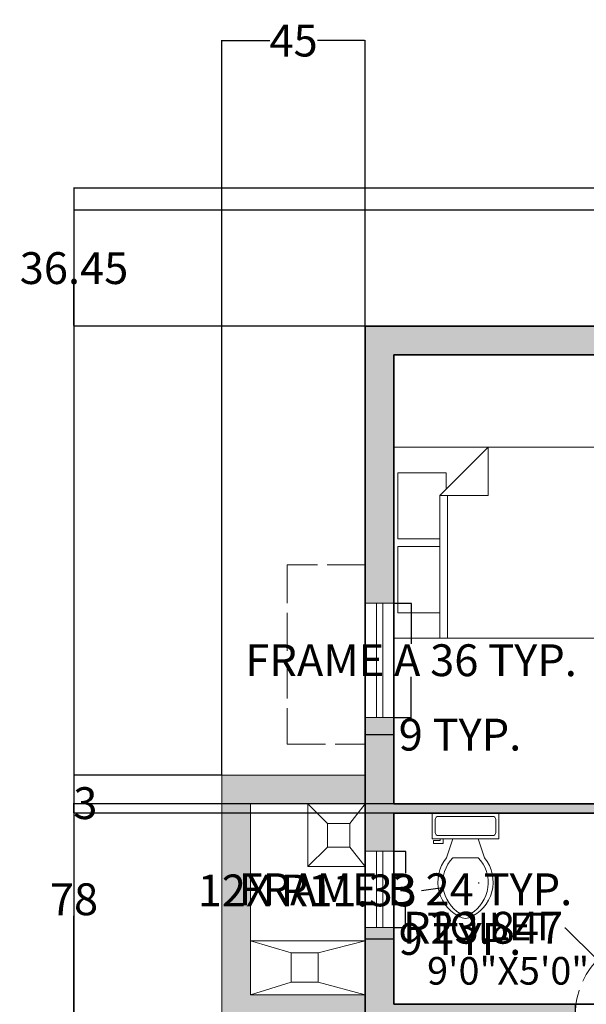
# Model space of a CAD drawing. Units: inches. Extents: x 215 to 969, y -612 to 418.
# Tile 5 of 8: x 227 to 405, y 109 to 418. Entities that reach past the tile are written whole.
import ezdxf

# ---------------------------------------------------------------- set-up
doc = ezdxf.new("R2010")
doc.units = ezdxf.units.IN
doc.header["$MEASUREMENT"] = 0
doc.linetypes.add('ACAD_ISO02W100', pattern=[15, 12, -3])
for name, color, linetype, lineweight in [('A-ANNO-DIMS', 2, 'Continuous', 18), ('A-AREA-IDEN', 7, 'Continuous', 18), ('A-DOOR', 3, 'Continuous', 25), ('A-DOOR-SWNG', 3, 'ACAD_ISO02W100', 13), ('A-FLOR-FIXT', 9, 'Continuous', 18), ('A-FLOR-OVHD', 8, 'ACAD_ISO02W100', 13), ('A-FLOR-SHFT', 9, 'Continuous', 18), ('A-FURN', 8, 'Continuous', 18), ('A-GLAZ', 4, 'Continuous', 18), ('A-WALL', 7, 'Continuous', 35)]:
    doc.layers.add(name, color=color, linetype=linetype, lineweight=lineweight)
doc.layers.add('A-WALL-PATT', color=252, linetype='Continuous', lineweight=13, true_color=0x939598)
doc.styles.get("Standard").update_dxf_attribs({"font": 'arial.ttf'})
doc.dimstyles.get("Standard").update_dxf_attribs({"dimtxt": 10, "dimasz": 0.18, "dimexe": 0.18, "dimexo": 0.0625, "dimgap": 0.09, "dimtad": 0, "dimtih": 1, "dimtoh": 1, "dimdec": 0, "dimzin": 0, "dimdsep": 46, "dimlunit": 3, "dimtxsty": 'Standard', "dimcen": 0.09, "dimadec": 0, "dimazin": 0, "dimtfac": 1, "dimtdec": 0, "dimtofl": 0, "dimtmove": 0, "dimatfit": 3, "dimfxl": 1, "dimtolj": 1, "dimtzin": 0, "dimarcsym": 0})

# ---------------------------------------------------------------- blocks, each defined once
blk = doc.blocks.new('Bed - Queen')
for p, q in [((0, -80.00003), (0, 0)), ((0, 0), (59.99999, 0)), ((59.99999, 0), (59.99999, -80.00003)), ((7.99999, -1.2), (28.79998, -1.2)), ((7.99999, -14.4), (7.99999, -1.2)), ((28.79998, -1.2), (28.79998, -14.4)), ((31.19999, -1.2), (51.99999, -1.2)), ((31.19999, -14.4), (31.19999, -1.2)), ((51.99999, -1.2), (51.99999, -16.4)), ((0, -14.4), (44.8, -14.4)), ((59.99999, -29.6), (44.8, -14.4)), ((44.8, -14.4), (44.8, -29.6)), ((44.8, -16.8), (0, -16.8)), ((51.99999, -16.4), (46.79936, -16.4)), ((44.8, -29.6), (59.99999, -29.6)), ((59.99999, -80.00003), (0, -80.00003))]:
    blk.add_line(p, q)
blk = doc.blocks.new('Toilet - top')
for p, q in [((9.5, -6), (9.5, -2)), ((-10, -8.5), (-8, -8.5)), ((-10, -9.5), (-10, -8.5)), ((-8, -8.5), (-8, -8)), ((-7, -8), (-7, -9.5)), ((-4, -8), (-6, -14)), ((4, -8), (6, -14)), ((-7, -9.5), (-10, -9.5)), ((4, -14), (-4, -14))]:
    blk.add_line(p, q)
blk.add_lwpolyline([(10.5, -8), (10.5, 0), (-10.5, 0), (-10.5, -8)], close=True)
for points in [[(-9.5, -2), (-9.5, -6)], [(8.5, -1), (-8.5, -1)], [(-8.5, -7), (8.5, -7)]]:
    blk.add_lwpolyline(points)
for centre, radius, start, end in [((-8.62, -1.88), 0.884, 81.8699, 188.1301), ((8.62, -1.88), 0.884, 351.8699, 98.1301), ((-8.62, -6.12), 0.884, 171.8699, 278.1301), ((8.62, -6.12), 0.884, 261.8699, 8.1301), ((3.52, -21.58), 12.17, 141.4691, 247.9714), ((4.2, -21.82), 11.33, 136.3677, 238.9468), ((-3.52, -21.58), 12.17, 292.0284, 38.5307), ((-4.2, -21.82), 11.33, 301.053, 43.6321), ((0, -27.88), 4, 245.7318, 294.2682), ((0, -29), 4, 254.8605, 285.1395)]:
    blk.add_arc(centre, radius, start, end)
blk = doc.blocks.new('WINDOW-SHADE-56')
for p, q in [((24.46, 56.34), (0, 56.34)), ((0, 56.34), (0, 0)), ((0, 0), (24.46, 0))]:
    blk.add_line(p, q)
blk = doc.blocks.new('WIN-FRAME-24B')
for p, q in [((0, 23.99), (9, 23.99)), ((3.5, 23.99), (3.5, 0)), ((5.5, 23.99), (5.5, 0)), ((9, 0), (0, 0)), ((4.5, 0), (9, 0))]:
    blk.add_line(p, q)
blk = doc.blocks.new('WIN-FRAME-36A')
for p, q in [((0, 35.94), (9, 35.94)), ((3.5, 35.94), (3.5, 0)), ((5.5, 35.94), (5.5, 0)), ((9, 0), (0, 0)), ((4.5, 0), (9, 0))]:
    blk.add_line(p, q)
blk = doc.blocks.new('*D41')
at = {"layer": 'A-ANNO-DIMS', "color": 0, "lineweight": -2, "transparency": 16777216}
for p, q in [((344.42, 235.25), (349.92, 235.25)), ((349.74, 235.07), (349.74, 222.48)), ((349.74, 199.49), (349.74, 212.08)), ((344.42, 199.31), (349.92, 199.31))]:
    blk.add_line(p, q, dxfattribs=at)
at = {"layer": 'A-ANNO-DIMS', "color": 0, "transparency": 16777216}
for points in [[(349.71, 235.07), (349.77, 235.07), (349.74, 235.25)], [(349.71, 199.49), (349.77, 199.49), (349.74, 199.31)]]:
    blk.add_solid(points, dxfattribs=at)
at = {"layer": 'Defpoints', "color": 0, "transparency": 16777216}
for p in [(344.35, 235.25), (349.74, 235.25), (344.35, 199.31)]:
    blk.add_point(p, dxfattribs=at)
at = {"layer": 'A-ANNO-DIMS', "color": 0, "transparency": 16777216, "insert": (349.74, 217.28), "char_height": 10, "attachment_point": 5}
blk.add_mtext('\\A1;FRAME A 36 TYP.', dxfattribs=at)
blk = doc.blocks.new('*D42')
at = {"layer": 'A-ANNO-DIMS', "color": 0, "lineweight": -2, "transparency": 16777216}
for p, q in [((335.35, 199.25), (335.35, 193.74)), ((344.35, 199.25), (344.35, 193.74)), ((335.53, 193.92), (344.17, 193.92)), ((344.35, 193.92), (344.53, 193.92))]:
    blk.add_line(p, q, dxfattribs=at)
at = {"layer": 'A-ANNO-DIMS', "color": 0, "transparency": 16777216}
for points in [[(335.53, 193.95), (335.53, 193.89), (335.35, 193.92)], [(344.17, 193.95), (344.17, 193.89), (344.35, 193.92)]]:
    blk.add_solid(points, dxfattribs=at)
at = {"layer": 'Defpoints', "color": 0, "transparency": 16777216}
for p in [(335.35, 199.31), (344.35, 199.31), (344.35, 193.92)]:
    blk.add_point(p, dxfattribs=at)
at = {"layer": 'A-ANNO-DIMS', "color": 0, "transparency": 16777216, "insert": (365.08, 193.92), "char_height": 10, "attachment_point": 5}
blk.add_mtext('\\A1;9 TYP.', dxfattribs=at)
blk = doc.blocks.new('*D47')
at = {"layer": 'A-ANNO-DIMS', "color": 0, "lineweight": -2, "transparency": 16777216}
for p, q in [((344.42, 157.34), (348.13, 157.34)), ((347.95, 157.16), (347.95, 150.45)), ((347.95, 133.52), (347.95, 140.23)), ((344.42, 133.34), (348.13, 133.34))]:
    blk.add_line(p, q, dxfattribs=at)
at = {"layer": 'A-ANNO-DIMS', "color": 0, "transparency": 16777216}
for points in [[(347.92, 157.16), (347.98, 157.16), (347.95, 157.34)], [(347.92, 133.52), (347.98, 133.52), (347.95, 133.34)]]:
    blk.add_solid(points, dxfattribs=at)
at = {"layer": 'Defpoints', "color": 0, "transparency": 16777216}
for p in [(344.35, 157.34), (347.95, 157.34), (344.35, 133.34)]:
    blk.add_point(p, dxfattribs=at)
at = {"layer": 'A-ANNO-DIMS', "color": 0, "transparency": 16777216, "insert": (347.95, 145.34), "char_height": 10, "attachment_point": 5}
blk.add_mtext('\\A1;FRAME B 24 TYP.', dxfattribs=at)
blk = doc.blocks.new('*D48')
at = {"layer": 'A-ANNO-DIMS', "color": 0, "lineweight": -2, "transparency": 16777216}
for p, q in [((335.35, 133.28), (335.35, 129.57)), ((344.35, 133.28), (344.35, 129.57)), ((335.53, 129.75), (344.17, 129.75)), ((344.35, 129.75), (344.53, 129.75))]:
    blk.add_line(p, q, dxfattribs=at)
at = {"layer": 'A-ANNO-DIMS', "color": 0, "transparency": 16777216}
for points in [[(335.53, 129.78), (335.53, 129.72), (335.35, 129.75)], [(344.17, 129.78), (344.17, 129.72), (344.35, 129.75)]]:
    blk.add_solid(points, dxfattribs=at)
at = {"layer": 'Defpoints', "color": 0, "transparency": 16777216}
for p in [(335.35, 133.34), (344.35, 133.34), (344.35, 129.75)]:
    blk.add_point(p, dxfattribs=at)
at = {"layer": 'A-ANNO-DIMS', "color": 0, "transparency": 16777216, "insert": (365.08, 129.75), "char_height": 10, "attachment_point": 5}
blk.add_mtext('\\A1;9 TYP.', dxfattribs=at)
blk = doc.blocks.new('*D73')
at = {"layer": 'A-ANNO-DIMS', "color": 0, "lineweight": -2, "transparency": 16777216}
for p, q in [((290.35, 181.28), (290.35, 412.08)), ((290.53, 411.9), (305.36, 411.9)), ((335.17, 411.9), (320.34, 411.9)), ((335.35, 181.28), (335.35, 412.08))]:
    blk.add_line(p, q, dxfattribs=at)
at = {"layer": 'A-ANNO-DIMS', "color": 0, "transparency": 16777216}
for points in [[(290.53, 411.93), (290.53, 411.87), (290.35, 411.9)], [(335.17, 411.93), (335.17, 411.87), (335.35, 411.9)]]:
    blk.add_solid(points, dxfattribs=at)
at = {"layer": 'Defpoints', "color": 0, "transparency": 16777216}
for p in [(335.35, 411.9), (290.35, 181.21), (335.35, 181.21)]:
    blk.add_point(p, dxfattribs=at)
at = {"layer": 'A-ANNO-DIMS', "color": 0, "transparency": 16777216, "insert": (312.85, 411.9), "char_height": 10, "attachment_point": 5}
blk.add_mtext('\\A1;45', dxfattribs=at)
blk = doc.blocks.new('*D74')
at = {"layer": 'A-ANNO-DIMS', "color": 0, "lineweight": -2, "transparency": 16777216}
for p, q in [((290.29, 181.21), (243.77, 181.21)), ((243.95, 181.03), (243.95, 147.41)), ((243.95, 103.39), (243.95, 137.02)), ((290.29, 103.21), (243.77, 103.21))]:
    blk.add_line(p, q, dxfattribs=at)
at = {"layer": 'A-ANNO-DIMS', "color": 0, "transparency": 16777216}
for points in [[(243.92, 181.03), (243.98, 181.03), (243.95, 181.21)], [(243.92, 103.39), (243.98, 103.39), (243.95, 103.21)]]:
    blk.add_solid(points, dxfattribs=at)
at = {"layer": 'Defpoints', "color": 0, "transparency": 16777216}
for p in [(243.95, 181.21), (290.35, 181.21), (290.35, 103.21)]:
    blk.add_point(p, dxfattribs=at)
at = {"layer": 'A-ANNO-DIMS', "color": 0, "transparency": 16777216, "insert": (243.95, 142.21), "char_height": 10, "attachment_point": 5}
blk.add_mtext('\\A1;78', dxfattribs=at)
blk = doc.blocks.new('*D76')
at = {"layer": 'A-ANNO-DIMS', "color": 0, "lineweight": -2, "transparency": 16777216}
for p, q in [((569.29, 365.5), (243.77, 365.5)), ((243.95, 365.32), (243.95, -91.71)), ((243.95, -559.13), (243.95, -102.1)), ((454.66, -559.31), (243.77, -559.31))]:
    blk.add_line(p, q, dxfattribs=at)
at = {"layer": 'A-ANNO-DIMS', "color": 0, "transparency": 16777216}
for points in [[(243.92, 365.32), (243.98, 365.32), (243.95, 365.5)], [(243.92, -559.13), (243.98, -559.13), (243.95, -559.31)]]:
    blk.add_solid(points, dxfattribs=at)
at = {"layer": 'Defpoints', "color": 0, "transparency": 16777216}
for p in [(569.35, 365.5), (243.95, -559.31), (454.72, -559.31)]:
    blk.add_point(p, dxfattribs=at)
at = {"layer": 'A-ANNO-DIMS', "color": 0, "transparency": 16777216, "insert": (243.95, -96.91), "char_height": 10, "attachment_point": 5}
blk.add_mtext('\\A1;924.8', dxfattribs=at)
blk = doc.blocks.new('*D78')
at = {"layer": 'A-ANNO-DIMS', "color": 0, "lineweight": -2, "transparency": 16777216}
for p, q in [((503.29, 358.66), (243.77, 358.66)), ((243.95, 358.48), (243.95, 345.64)), ((243.95, 322.39), (243.95, 335.24)), ((503.29, 322.21), (243.77, 322.21))]:
    blk.add_line(p, q, dxfattribs=at)
at = {"layer": 'A-ANNO-DIMS', "color": 0, "transparency": 16777216}
for points in [[(243.92, 358.48), (243.98, 358.48), (243.95, 358.66)], [(243.92, 322.39), (243.98, 322.39), (243.95, 322.21)]]:
    blk.add_solid(points, dxfattribs=at)
at = {"layer": 'Defpoints', "color": 0, "transparency": 16777216}
for p in [(503.35, 358.66), (243.95, 322.21), (503.35, 322.21)]:
    blk.add_point(p, dxfattribs=at)
at = {"layer": 'A-ANNO-DIMS', "color": 0, "transparency": 16777216, "insert": (243.95, 340.44), "char_height": 10, "attachment_point": 5}
blk.add_mtext('\\A1;36.45', dxfattribs=at)
blk = doc.blocks.new('*D83')
at = {"layer": 'A-ANNO-DIMS', "color": 0, "lineweight": -2, "transparency": 16777216}
for p, q in [((344.29, 172.21), (243.77, 172.21)), ((243.95, 172.21), (243.95, 172.39)), ((243.95, 172.39), (244.13, 172.39)), ((243.95, 169.39), (243.95, 172.03)), ((344.29, 169.21), (243.77, 169.21))]:
    blk.add_line(p, q, dxfattribs=at)
at = {"layer": 'A-ANNO-DIMS', "color": 0, "transparency": 16777216}
for points in [[(243.92, 172.03), (243.98, 172.03), (243.95, 172.21)], [(243.92, 169.39), (243.98, 169.39), (243.95, 169.21)]]:
    blk.add_solid(points, dxfattribs=at)
at = {"layer": 'Defpoints', "color": 0, "transparency": 16777216}
for p in [(243.95, 172.21), (344.35, 172.21), (344.35, 169.21)]:
    blk.add_point(p, dxfattribs=at)
at = {"layer": 'A-ANNO-DIMS', "color": 0, "transparency": 16777216, "insert": (247.5, 172.39), "char_height": 10, "attachment_point": 5}
blk.add_mtext('\\A1;3', dxfattribs=at)
blk = doc.blocks.new('*D85')
at = {"layer": 'A-ANNO-DIMS', "color": 0, "lineweight": -2, "transparency": 16777216}
for p, q in [((397.96, 133.26), (398.14, 133.26)), ((398.14, 133.26), (408.16, 123.3)), ((425.11, 106.37), (425.29, 106.37)), ((425.2, 106.28), (425.2, 106.46))]:
    blk.add_line(p, q, dxfattribs=at)
at = {"layer": 'A-ANNO-DIMS', "color": 0, "transparency": 16777216}
blk.add_solid([(408.18, 123.32), (408.14, 123.28), (408.29, 123.18)], dxfattribs=at)
at = {"layer": 'Defpoints', "color": 0, "transparency": 16777216}
for p in [(408.29, 123.18), (425.2, 106.37)]:
    blk.add_point(p, dxfattribs=at)
at = {"layer": 'A-ANNO-DIMS', "color": 0, "transparency": 16777216, "insert": (372.32, 133.26), "char_height": 10, "attachment_point": 5}
blk.add_mtext('\\A1;R23.847', dxfattribs=at)
blk = doc.blocks.new('*D96')
at = {"layer": 'A-ANNO-DIMS', "color": 0, "lineweight": -2, "transparency": 16777216}
for p, q in [((353.05, 144.98), (359.61, 145.86)), ((370.93, 147.4), (371.11, 147.4)), ((371.02, 147.31), (371.02, 147.49))]:
    blk.add_line(p, q, dxfattribs=at)
at = {"layer": 'A-ANNO-DIMS', "color": 0, "transparency": 16777216}
blk.add_solid([(359.61, 145.89), (359.62, 145.83), (359.79, 145.88)], dxfattribs=at)
at = {"layer": 'Defpoints', "color": 0, "transparency": 16777216}
for p in [(359.79, 145.88), (371.02, 147.4)]:
    blk.add_point(p, dxfattribs=at)
at = {"layer": 'A-ANNO-DIMS', "color": 0, "transparency": 16777216, "insert": (317.15, 144.98), "char_height": 10, "attachment_point": 5}
blk.add_mtext('\\A1;12X R11.33', dxfattribs=at)

msp = doc.modelspace()

# ---------------------------------------------------------------- hatches: boundary and pattern name
at = {"layer": 'A-WALL-PATT'}
h = msp.add_hatch(color=256, dxfattribs=at)
h.dxf.hatch_style = 1
h.paths.add_polyline_path([(764.0736, 322.2135), (569.3535, 322.2135), (565.0643, 322.2135), (565.0643, 313.2135), (569.3535, 313.2135), (569.3535, 205.2135), (509.3535, 205.2135), (509.3535, 247.2592), (506.3535, 247.2592), (506.3535, 172.2135), (491.3535, 172.2135), (491.3535, 169.2135), (509.3535, 169.2135), (509.3535, 202.2135), (569.3535, 202.2135), (569.3535, 169.2135), (578.3535, 169.2135), (578.3535, 205.2135), (578.3535, 237.2135), (615.7789, 237.2135), (615.7789, 246.2135), (578.3535, 246.2135), (578.3535, 313.2135), (710.3535, 313.2135), (710.3535, 246.2135), (710.3535, 211.3874), (719.3535, 211.3874), (719.3535, 295.2135), (719.3535, 313.2135), (764.0736, 313.2135)])
h.paths.add_polyline_path([(879.3535, 322.2135), (811.6486, 322.2135), (811.6486, 313.2135), (870.3535, 313.2135), (870.3535, 215.3905, -0.06325422), (879.3535, 216.5337), (879.3535, 313.2135)])
h.paths.add_polyline_path([(879.3535, 157.2135), (879.3535, 180.5337), (870.3535, 180.5337), (870.3535, 157.2135), (719.3535, 157.2135), (710.3535, 157.2135), (710.3535, 148.2135), (719.3535, 148.2135), (870.3535, 148.2135), (870.3535, 16.2135), (838.4933, 16.2135), (838.4933, 13.2135), (870.3535, 13.2135), (870.3535, -37.7865), (844.0345, -37.7865), (844.0345, -46.7865), (870.3535, -46.7865), (879.3535, -46.7865), (879.3535, -37.7865), (879.3535, 137.613)])
h.paths.add_polyline_path([(710.3535, 246.2135), (663.4146, 246.2135), (663.4146, 237.2135), (710.3535, 237.2135)], flags=17)
h.paths.add_polyline_path([(541.2942, 322.2135), (509.3535, 322.2135), (468.3222, 322.2135), (468.3222, 313.2135), (500.3535, 313.2135), (509.3535, 313.2135), (541.2942, 313.2135)])
h.paths.add_polyline_path([(509.3535, 313.2135), (503.3535, 313.2135), (503.3535, 277.5241, -0.04952579), (509.3535, 277.4203)], flags=17)
h.paths.add_polyline_path([(420.2828, 322.2135), (335.3535, 322.2135), (335.3535, 235.2487), (344.3535, 235.2487), (344.3535, 284.1885), (344.3535, 313.2135), (420.2828, 313.2135)])
h.paths.add_polyline_path([(335.3535, 181.2135), (290.3535, 181.2135), (290.3535, 103.2135), (335.3535, 103.2135), (335.3535, 112.2135), (299.3535, 112.2135), (299.3535, 129.1615), (299.3535, 172.2135), (335.3535, 172.2135)])
h.paths.add_polyline_path([(344.3535, 199.3097), (335.3535, 199.3097), (335.3535, 172.2135), (335.3535, 157.3369), (344.3535, 157.3369), (344.3535, 169.2135), (452.3535, 169.2135), (452.5037, 169.2135), (452.5037, 150.1199), (452.3535, 109.2135), (455.3535, 109.2135), (455.3535, 169.2135, -0.02086055), (455.4787, 172.2135), (344.3535, 172.2135)])
h.paths.add_polyline_path([(344.3535, 133.3441), (335.3535, 133.3441), (335.3535, 77.89), (344.3535, 77.89), (344.3535, 103.2135), (401.3556, 103.2135), (401.3556, 109.2135), (344.3535, 109.2135)])
h.paths.add_polyline_path([(462.6362, 109.2135), (443.0437, 109.2135), (425.2018, 109.2135), (425.2018, 106.2135), (452.3535, 106.2135), (462.7615, 106.2135, -0.02086055)])
h.paths.add_polyline_path([(540.3535, 106.2135), (684.3535, 106.2135), (684.3535, 35.7135), (687.3535, 35.7135), (687.3535, 56.1856), (693.3535, 56.1856), (693.3535, 109.2135), (540.3535, 109.2135), (531.3535, 109.2135), (498.6362, 109.2135), (498.6362, 106.2135), (531.3535, 106.2135), (531.3535, -37.7865), (507.9524, -37.7865), (507.9524, -46.7865), (610.6038, -46.7865), (610.6038, -37.7865), (540.3535, -37.7865)])
h.paths.add_polyline_path([(578.3535, 358.6622), (555.879, 358.6622), (555.879, 349.6622), (569.3535, 349.6622), (569.3535, 322.2135), (578.3535, 322.2135)])
h.paths.add_polyline_path([(525.962, 358.6622), (503.3535, 358.6622), (503.3535, 322.2135), (509.3535, 322.2135), (509.3535, 349.6622), (525.962, 349.6622)])
h.paths.add_polyline_path([(344.3535, 30.022), (335.3535, 30.022), (335.3535, -37.7865), (335.3535, -46.7865), (484.3302, -46.7865), (484.3302, -37.7865), (344.3535, -37.7865)])
h.paths.add_polyline_path([(719.1188, -37.7865), (698.4193, -37.7865), (693.3535, -37.7865), (693.3535, 7.424, -0.07717369), (684.3535, 6.0404), (684.3535, -37.7865), (658.8269, -37.7865), (658.8269, -46.7865), (684.3535, -46.7865), (684.3535, -82.7865), (693.3535, -82.7865), (704.1236, -82.7865), (704.1236, -78.0462), (693.3535, -78.0462), (693.3535, -46.7865), (719.1188, -46.7865)])
h.paths.add_polyline_path([(684.3535, -14.2202), (669.6716, -14.2202), (669.6716, -16.6044, -0.23606798), (667.6716, -17.6044), (667.6716, -18.6044, -0.11764706), (650.6716, -18.6044), (650.6716, -17.6044, -0.23606798), (648.6716, -16.6044), (648.6716, -14.2202), (603.0565, -14.2202), (603.0565, -37.7865), (684.3535, -37.7865)], flags=17)
h.paths.add_polyline_path([(665.6716, -14.2202), (652.6716, -14.2202), (652.6716, -16.6044, -0.23606798), (650.6716, -17.6044), (650.6716, -18.6044, 0.11764706), (667.6716, -18.6044), (667.6716, -17.6044, -0.23606798), (665.6716, -16.6044)], flags=16)
h.paths.add_polyline_path([(786.7385, -37.7865), (755.3535, -37.7865), (755.3535, 13.2135), (769.0808, 13.2135), (769.0808, 16.2135), (755.3535, 16.2135), (755.3535, 73.2135), (753.3535, 73.2135), (693.3535, 73.2135), (693.3535, 70.2135), (753.3535, 70.2135), (753.3535, -37.7865), (743.3062, -37.7865), (743.3062, -46.7865), (781.7385, -46.7865), (781.7385, -82.7865), (786.7385, -82.7865), (786.7385, -82.3744), (786.7385, -46.7865)])
h.paths.add_polyline_path([(844.0345, -37.7865), (786.7385, -37.7865), (786.7385, -46.7865), (844.0345, -46.7865)], flags=17)
h.paths.add_polyline_path([(781.7385, -78.0462), (704.1236, -78.0462), (704.1236, -82.7865), (781.7385, -82.7865)], flags=17)
h.paths.add_polyline_path([(344.3535, -46.7865), (335.3535, -46.7865), (335.3535, -166.4525), (344.3535, -166.4525)])
h.paths.add_polyline_path([(382.6632, 103.2135), (344.3535, 103.2135), (344.3535, 77.89), (344.3535, 32.7135), (363.5083, 32.7135), (382.6632, 32.7135)])
h.paths.add_polyline_path([(879.3535, -46.7865), (870.3535, -46.7865), (870.3535, -166.4525), (879.3535, -166.4525)])
h.paths.add_polyline_path([(879.3535, -166.4525), (799.4745, -166.4525), (799.4745, -175.4525), (855.3535, -175.4525), (870.3535, -175.4525), (870.3535, -192.5449), (879.3535, -192.5449), (879.3535, -175.4525)])
h.paths.add_polyline_path([(763.1775, -166.4525), (655.7214, -166.4525), (655.7214, -175.4525), (763.1775, -175.4525)])
h.paths.add_polyline_path([(619.8538, -166.4525), (550.8369, -166.4525), (550.8369, -175.4525), (619.8538, -175.4525)])
h.paths.add_polyline_path([(527.1282, -166.4525), (427.0819, -166.4525), (427.0819, -175.4525), (527.1282, -175.4525)])
h.paths.add_polyline_path([(391.4021, -166.4525), (335.3535, -166.4525), (335.3535, -175.4525), (335.3535, -236.0109), (344.3535, -236.0109), (344.3535, -187.5037), (344.3535, -175.4525), (391.4021, -175.4525)])
h.paths.add_polyline_path([(344.3535, -271.9249), (335.3535, -271.9249), (335.3535, -331.0209), (344.3535, -331.0209), (344.3535, -314.4525), (412.4218, -314.4525, -0.02503209), (412.3073, -311.4525), (344.3535, -311.4525)])
h.paths.add_polyline_path([(470.1954, -311.4525), (442.3073, -311.4525), (442.3073, -314.4525), (470.0702, -314.4525, -0.02086055)])
h.paths.add_polyline_path([(455.3535, -314.4525), (452.3535, -314.4525), (452.3535, -374.4525), (455.3535, -374.4525)])
h.paths.add_polyline_path([(579.3535, -241.4072), (519.3535, -241.4072), (519.3535, -283.4525), (579.3535, -283.4525)])
h.paths.add_polyline_path([(516.5043, -281.1089), (584.3098, -281.1089), (584.3098, -264.0138), (516.5043, -264.0138)], flags=9)
h.paths.add_polyline_path([(516.4662, -263.2183), (581.1504, -263.2183), (581.1504, -245.8948), (516.4662, -245.8948)], flags=9)

# ---------------------------------------------------------------- linework, layer by layer
at = {"layer": 'A-DOOR'}
msp.add_line((401.3556, 103.2135), (401.3556, 109.2135), dxfattribs=at)
at = {"layer": 'A-DOOR-SWNG'}
msp.add_arc((425.2018, 106.3669), 23.8466, 90, 180.368506, dxfattribs=at)
at = {"layer": 'A-FLOR-SHFT'}
for p, q in [((290.3535, 181.2135), (290.3535, 103.2135)), ((335.3535, 181.2135), (290.3535, 181.2135)), ((335.3535, 172.2135), (299.3535, 172.2135)), ((299.3535, 172.2135), (299.3535, 112.2135)), ((323.4787, 166.0316), (317.3245, 172.2135)), ((330.538, 166.0316), (335.3535, 172.2135)), ((323.4787, 158.6192), (317.3245, 152.4723)), ((330.538, 158.6192), (335.3535, 152.4723)), ((312.1553, 125.4125), (299.3535, 129.1615)), ((320.5486, 125.4125), (335.3535, 129.1615)), ((312.1553, 116.1621), (299.3535, 112.2135)), ((320.5486, 116.1621), (335.3535, 112.2135)), ((299.3535, 112.2135), (335.3535, 112.2135))]:
    msp.add_line(p, q, dxfattribs=at)
for points in [[(335.3535, 172.2135), (317.3245, 172.2135), (317.3245, 152.4723), (335.3535, 152.4723)], [(323.4787, 166.0316), (330.538, 166.0316), (330.538, 158.6192), (323.4787, 158.6192)], [(335.3535, 112.2135), (299.3535, 112.2135), (299.3535, 129.1615), (335.3535, 129.1615)], [(312.1553, 125.4125), (320.5486, 125.4125), (320.5486, 116.1621), (312.1553, 116.1621)]]:
    msp.add_lwpolyline(points, close=True, dxfattribs=at)
at = {"layer": 'A-WALL'}
for p, q in [((335.3535, 322.2135), (509.3535, 322.2135)), ((335.3535, 322.2135), (335.3535, 172.2135)), ((344.3535, 313.2135), (500.3535, 313.2135)), ((344.3535, 313.2135), (344.3535, 172.2135)), ((335.3535, -37.7865), (335.3535, 172.2135)), ((344.3535, 172.2135), (455.4787, 172.2135)), ((335.3535, 169.2135), (335.3535, 109.2135)), ((344.3535, 169.2135), (452.3535, 169.2135)), ((344.3535, 169.2135), (344.3535, 109.2135)), ((344.3535, 109.2135), (452.3535, 109.2135))]:
    msp.add_line(p, q, dxfattribs=at)

# ---------------------------------------------------------------- block references
at = {"layer": 'A-FLOR-FIXT'}
msp.add_blockref('Toilet - top', (366.8192, 169.2135), dxfattribs=at)
at = {"layer": 'A-FLOR-OVHD'}
msp.add_blockref('WINDOW-SHADE-56', (310.895, 190.878), dxfattribs=at)
at = {"layer": 'A-FURN', "rotation": 90}
msp.add_blockref('Bed - Queen', (344.3535, 224.1885), dxfattribs=at)
at = {"layer": 'A-GLAZ'}
for name, p in [('WIN-FRAME-36A', (335.353, 199.31)), ('WIN-FRAME-24B', (335.353, 133.344))]:
    msp.add_blockref(name, p, dxfattribs=at)

# ---------------------------------------------------------------- texts
at = {"layer": 'A-AREA-IDEN'}
for s, p in [('TOILET', (354.7688, 129.3376)), ('9\'0"X5\'0"', (354.7688, 115.3982))]:
    msp.add_text(s, height=8.67737, dxfattribs=at).set_placement(p)

# ---------------------------------------------------------------- dimensions: what is measured, and where the dimension line sits
at = {"layer": 'A-ANNO-DIMS'}
dim = msp.add_linear_dim(base=(335.3535, 411.9008), p1=(290.3535, 181.2135), p2=(335.3535, 181.2135), dimstyle='Standard', override={"dimdec": 0, "dimlfac": 1, "dimrnd": 0, "dimzin": 0, "dimdsep": 46, "dimlunit": 2}, dxfattribs=at)
dim.commit()
dim.dimension.update_dxf_attribs({"geometry": '*D73', "text_midpoint": (312.8535, 411.9008)})
for base, p1, p2, override, picture, middle in [((243.9535, -559.3132), (569.3535, 365.5008), (454.7218, -559.3132), {"dimdec": 1, "dimlfac": 1, "dimrnd": 0, "dimzin": 0, "dimdsep": 46, "dimlunit": 2}, '*D76', (243.9535, -96.9062)), ((243.9535, 322.2135), (503.3535, 358.6622), (503.3535, 322.2135), {"dimdec": 2, "dimlfac": 1, "dimrnd": 0, "dimzin": 0, "dimdsep": 46, "dimlunit": 2}, '*D78', (243.9535, 340.4379)), ((243.9535, 181.2135), (290.3535, 103.2135), (290.3535, 181.2135), {"dimdec": 0, "dimlfac": 1, "dimrnd": 0, "dimzin": 0, "dimdsep": 46, "dimlunit": 2}, '*D74', (243.9535, 142.2135)), ((243.9535, 172.2135), (344.3535, 169.2135), (344.3535, 172.2135), {"dimdec": 0, "dimlfac": 1, "dimrnd": 0, "dimzin": 0, "dimdsep": 46, "dimlunit": 2}, '*D83', (247.4977, 172.3935))]:
    dim = msp.add_linear_dim(base=base, p1=p1, p2=p2, angle=90, dimstyle='Standard', override=override, dxfattribs=at)
    dim.commit()
    dim.dimension.update_dxf_attribs({"geometry": picture, "text_midpoint": middle})
for base, p1, p2, text, picture, middle in [((349.7443, 235.2487), (344.3535, 199.3097), (344.3535, 235.2487), 'FRAME A <> TYP.', '*D41', (349.7443, 217.2792)), ((347.9524, 157.3369), (344.3535, 133.3441), (344.3535, 157.3369), 'FRAME B <> TYP.', '*D47', (347.9524, 145.3405))]:
    dim = msp.add_linear_dim(base=base, p1=p1, p2=p2, angle=90, text=text, dimstyle='Standard', override={"dimdec": 0, "dimlfac": 1, "dimrnd": 0, "dimzin": 0, "dimdsep": 46, "dimlunit": 2}, dxfattribs=at)
    dim.commit()
    dim.dimension.update_dxf_attribs({"geometry": picture, "text_midpoint": middle})
for base, p1, p2, picture, middle in [((344.3535, 193.9188), (335.3535, 199.3097), (344.3535, 199.3097), '*D42', (365.0771, 193.9188)), ((344.3535, 129.7452), (335.3535, 133.3441), (344.3535, 133.3441), '*D48', (365.0771, 129.7452))]:
    dim = msp.add_linear_dim(base=base, p1=p1, p2=p2, text='<> TYP.', dimstyle='Standard', override={"dimdec": 0, "dimlfac": 1, "dimrnd": 0, "dimzin": 0, "dimdsep": 46, "dimlunit": 2}, dxfattribs=at)
    dim.commit()
    dim.dimension.update_dxf_attribs({"geometry": picture, "text_midpoint": middle})
dim = msp.add_radius_dim(center=(371.0192, 147.3961), mpoint=(359.7915, 145.8829), text='12X <>', dimstyle='Standard', override={"dimdec": 2, "dimlfac": 1, "dimrnd": 0, "dimzin": 0, "dimdsep": 46, "dimlunit": 2}, dxfattribs=at)
dim.commit()
dim.dimension.update_dxf_attribs({"geometry": '*D96', "text_midpoint": (353.0549, 144.975), "dimtype": 164})
dim = msp.add_radius_dim(center=(425.2018, 106.3669), mpoint=(408.2859, 123.1751), dimstyle='Standard', override={"dimdec": 3, "dimlfac": 1, "dimrnd": 0, "dimzin": 0, "dimdsep": 46, "dimlunit": 2}, dxfattribs=at)
dim.commit()
dim.dimension.update_dxf_attribs({"geometry": '*D85', "text_midpoint": (372.3241, 133.26), "dimtype": 164})

doc.saveas('drawing.dxf')
